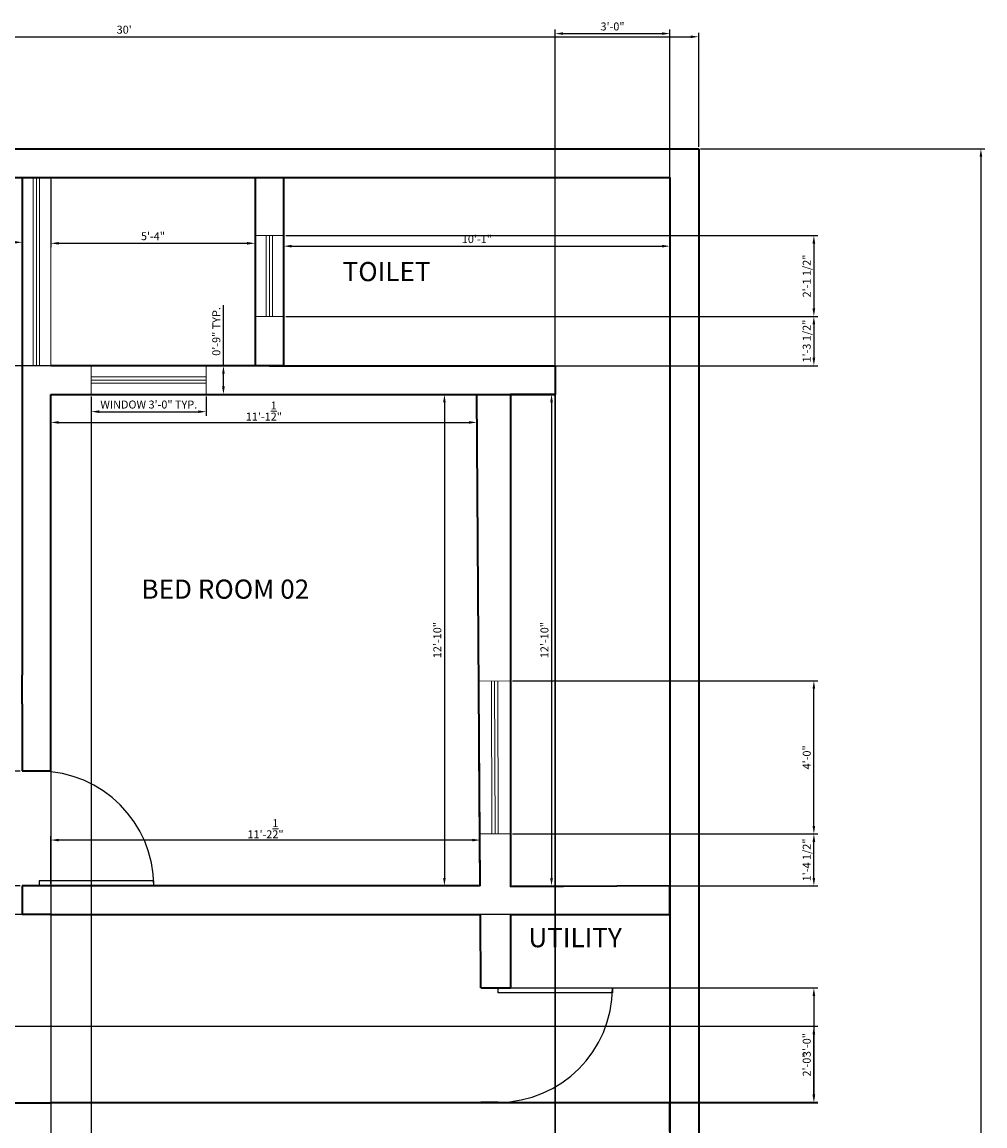
# Model space of a CAD drawing. Units: inches. Extents: x 2178 to 2667, y 1439 to 2239.
# Tile 5 of 5: x 2366 to 2667, y 1891 to 2237. Entities that reach past the tile are written whole.
import ezdxf

# ---------------------------------------------------------------- set-up
doc = ezdxf.new("R2010")
doc.units = ezdxf.units.IN
for name, color, linetype, lineweight in [('A-ANNO-DIMS', 2, 'Continuous', 18), ('A-AREA-IDEN', 7, 'Continuous', 18), ('A-DOOR', 3, 'Continuous', 25), ('A-GLAZ', 4, 'Continuous', 18), ('A-WALL', 7, 'Continuous', 35)]:
    doc.layers.add(name, color=color, linetype=linetype, lineweight=lineweight)
doc.styles.get("Standard").update_dxf_attribs({"font": 'arial.ttf'})
doc.dimstyles.new('Copy of ISO-25', dxfattribs={"dimtxt": 2.5, "dimasz": 2.5, "dimexe": 1.25, "dimexo": 0.625, "dimtad": 1, "dimdec": 1, "dimlunit": 4, "dimtxsty": 'Standard', "dimcen": 2.5, "dimadec": 0, "dimazin": 0, "dimtfac": 1, "dimtdec": 1, "dimtmove": 0, "dimatfit": 3, "dimfxl": 1, "dimarcsym": 0})

# ---------------------------------------------------------------- blocks, each defined once
blk = doc.blocks.new('*D1')
at = {"layer": 'A-ANNO-DIMS', "color": 0, "lineweight": -2, "transparency": 16777216}
for p, q in [((2226.53, 2187.41), (2226.53, 2166.47)), ((2365.53, 2187.41), (2365.53, 2166.47)), ((2229.03, 2167.72), (2363.03, 2167.72))]:
    blk.add_line(p, q, dxfattribs=at)
at = {"layer": 'A-ANNO-DIMS', "color": 0, "transparency": 16777216}
for points in [[(2229.03, 2168.13), (2229.03, 2167.3), (2226.53, 2167.72)], [(2363.03, 2168.13), (2363.03, 2167.3), (2365.53, 2167.72)]]:
    blk.add_solid(points, dxfattribs=at)
at = {"layer": 'Defpoints', "color": 0, "transparency": 16777216}
for p in [(2226.53, 2188.03), (2365.53, 2188.03), (2365.53, 2167.72)]:
    blk.add_point(p, dxfattribs=at)
at = {"layer": 'A-ANNO-DIMS', "color": 0, "transparency": 16777216, "insert": (2296.03, 2169.6), "char_height": 2.5, "attachment_point": 5}
blk.add_mtext('11\'-7"', dxfattribs=at)
blk = doc.blocks.new('*D2')
at = {"layer": 'A-ANNO-DIMS', "color": 0, "lineweight": -2, "transparency": 16777216}
for p, q in [((2374.53, 2187.41), (2374.53, 2166.16)), ((2438.53, 2187.41), (2438.53, 2166.16)), ((2377.03, 2167.41), (2436.03, 2167.41))]:
    blk.add_line(p, q, dxfattribs=at)
at = {"layer": 'A-ANNO-DIMS', "color": 0, "transparency": 16777216}
for points in [[(2377.03, 2167.83), (2377.03, 2166.99), (2374.53, 2167.41)], [(2436.03, 2167.83), (2436.03, 2166.99), (2438.53, 2167.41)]]:
    blk.add_solid(points, dxfattribs=at)
at = {"layer": 'Defpoints', "color": 0, "transparency": 16777216}
for p in [(2374.53, 2188.03), (2438.53, 2188.03), (2438.53, 2167.41)]:
    blk.add_point(p, dxfattribs=at)
at = {"layer": 'A-ANNO-DIMS', "color": 0, "transparency": 16777216, "insert": (2406.53, 2169.31), "char_height": 2.5, "attachment_point": 5}
blk.add_mtext('5\'-4"', dxfattribs=at)
blk = doc.blocks.new('*D3')
at = {"layer": 'A-ANNO-DIMS', "color": 0, "lineweight": -2, "transparency": 16777216}
for p, q in [((2447.53, 2187.41), (2447.53, 2165.26)), ((2568.53, 2187.41), (2568.53, 2165.26)), ((2450.03, 2166.51), (2566.03, 2166.51))]:
    blk.add_line(p, q, dxfattribs=at)
at = {"layer": 'A-ANNO-DIMS', "color": 0, "transparency": 16777216}
for points in [[(2450.03, 2166.93), (2450.03, 2166.09), (2447.53, 2166.51)], [(2566.03, 2166.93), (2566.03, 2166.09), (2568.53, 2166.51)]]:
    blk.add_solid(points, dxfattribs=at)
at = {"layer": 'Defpoints', "color": 0, "transparency": 16777216}
for p in [(2447.53, 2188.03), (2568.53, 2188.03), (2568.53, 2166.51)]:
    blk.add_point(p, dxfattribs=at)
at = {"layer": 'A-ANNO-DIMS', "color": 0, "transparency": 16777216, "insert": (2508.03, 2168.41), "char_height": 2.5, "attachment_point": 5}
blk.add_mtext('10\'-1"', dxfattribs=at)
blk = doc.blocks.new('*D6')
at = {"layer": 'A-ANNO-DIMS', "color": 0, "lineweight": -2, "transparency": 16777216}
for p, q in [((2374.53, 2119.41), (2374.53, 2110.02)), ((2508.03, 2119.41), (2508.03, 2110.02)), ((2377.03, 2111.27), (2505.53, 2111.27))]:
    blk.add_line(p, q, dxfattribs=at)
at = {"layer": 'A-ANNO-DIMS', "color": 0, "transparency": 16777216}
for points in [[(2377.03, 2111.69), (2377.03, 2110.86), (2374.53, 2111.27)], [(2505.53, 2111.69), (2505.53, 2110.86), (2508.03, 2111.27)]]:
    blk.add_solid(points, dxfattribs=at)
at = {"layer": 'Defpoints', "color": 0, "transparency": 16777216}
for p in [(2374.53, 2120.03), (2508.03, 2120.03), (2508.03, 2111.27)]:
    blk.add_point(p, dxfattribs=at)
at = {"layer": 'A-ANNO-DIMS', "color": 0, "transparency": 16777216, "insert": (2441.28, 2114.83), "char_height": 2.5, "attachment_point": 5}
blk.add_mtext('11\'-1{\\H1x;\\S1/2;}"', dxfattribs=at)
blk = doc.blocks.new('*D7')
at = {"layer": 'A-ANNO-DIMS', "color": 0, "lineweight": -2, "transparency": 16777216}
for p, q in [((2507.4, 2120.03), (2496.61, 2120.03)), ((2497.86, 2117.53), (2497.86, 1968.53)), ((2508.44, 1966.03), (2496.61, 1966.03))]:
    blk.add_line(p, q, dxfattribs=at)
at = {"layer": 'A-ANNO-DIMS', "color": 0, "transparency": 16777216}
for points in [[(2497.45, 2117.53), (2498.28, 2117.53), (2497.86, 2120.03)], [(2497.45, 1968.53), (2498.28, 1968.53), (2497.86, 1966.03)]]:
    blk.add_solid(points, dxfattribs=at)
at = {"layer": 'Defpoints', "color": 0, "transparency": 16777216}
for p in [(2508.03, 2120.03), (2497.86, 1966.03), (2509.07, 1966.03)]:
    blk.add_point(p, dxfattribs=at)
at = {"layer": 'A-ANNO-DIMS', "color": 0, "transparency": 16777216, "insert": (2495.96, 2043.03), "char_height": 2.5, "attachment_point": 5, "rotation": 90}
blk.add_mtext('12\'-10"', dxfattribs=at)
blk = doc.blocks.new('*D8')
at = {"layer": 'A-ANNO-DIMS', "color": 0, "lineweight": -2, "transparency": 16777216}
for p, q in [((2374.53, 1966.66), (2374.53, 1981.63)), ((2506.57, 1980.38), (2377.03, 1980.38)), ((2509.07, 1966.66), (2509.07, 1981.63))]:
    blk.add_line(p, q, dxfattribs=at)
at = {"layer": 'A-ANNO-DIMS', "color": 0, "transparency": 16777216}
for points in [[(2377.03, 1980.79), (2377.03, 1979.96), (2374.53, 1980.38)], [(2506.57, 1980.79), (2506.57, 1979.96), (2509.07, 1980.38)]]:
    blk.add_solid(points, dxfattribs=at)
at = {"layer": 'Defpoints', "color": 0, "transparency": 16777216}
for p in [(2374.53, 1980.38), (2374.53, 1966.03), (2509.07, 1966.03)]:
    blk.add_point(p, dxfattribs=at)
at = {"layer": 'A-ANNO-DIMS', "color": 0, "transparency": 16777216, "insert": (2441.8, 1983.93), "char_height": 2.5, "attachment_point": 5}
blk.add_mtext('11\'-2{\\H1x;\\S1/2;}"', dxfattribs=at)
blk = doc.blocks.new('*D9')
at = {"layer": 'A-ANNO-DIMS', "color": 0, "lineweight": -2, "transparency": 16777216}
for p, q in [((2519.15, 2120.03), (2532.68, 2120.03)), ((2531.43, 2117.53), (2531.43, 1968.53)), ((2519.15, 1966.03), (2532.68, 1966.03))]:
    blk.add_line(p, q, dxfattribs=at)
at = {"layer": 'A-ANNO-DIMS', "color": 0, "transparency": 16777216}
for points in [[(2531.01, 2117.53), (2531.85, 2117.53), (2531.43, 2120.03)], [(2531.01, 1968.53), (2531.85, 1968.53), (2531.43, 1966.03)]]:
    blk.add_solid(points, dxfattribs=at)
at = {"layer": 'Defpoints', "color": 0, "transparency": 16777216}
for p in [(2518.53, 2120.03), (2518.53, 1966.03), (2531.43, 1966.03)]:
    blk.add_point(p, dxfattribs=at)
at = {"layer": 'A-ANNO-DIMS', "color": 0, "transparency": 16777216, "insert": (2529.53, 2043.03), "char_height": 2.5, "attachment_point": 5, "rotation": 90}
blk.add_mtext('12\'-10"', dxfattribs=at)
blk = doc.blocks.new('*U23')
for p, q in [((-40, 0), (-40, 6)), ((0, 0), (0, 6))]:
    blk.add_line(p, q)
blk.add_lwpolyline([(0, 0), (0, -40), (-1.75, -40), (-1.75, 0)], close=True)
blk.add_arc((0, 0), 40, 180, 270)
blk = doc.blocks.new('*U22')
for p, q in [((0, 0), (0, 6)), ((40, 0), (40, 6))]:
    blk.add_line(p, q)
blk.add_lwpolyline([(0, 0), (0, -40), (1.75, -40), (1.75, 0)], close=True)
blk.add_arc((0, 0), 40, 270, 0)
blk = doc.blocks.new('*D37')
at = {"layer": 'A-ANNO-DIMS', "color": 0, "lineweight": -2, "transparency": 16777216}
for p, q in [((2364.9, 2001.92), (2358.2, 2001.92)), ((2359.45, 1999.42), (2359.45, 1968.53)), ((2364.9, 1966.03), (2358.2, 1966.03))]:
    blk.add_line(p, q, dxfattribs=at)
at = {"layer": 'A-ANNO-DIMS', "color": 0, "transparency": 16777216}
for points in [[(2359.04, 1999.42), (2359.87, 1999.42), (2359.45, 2001.92)], [(2359.04, 1968.53), (2359.87, 1968.53), (2359.45, 1966.03)]]:
    blk.add_solid(points, dxfattribs=at)
at = {"layer": 'Defpoints', "color": 0, "transparency": 16777216}
for p in [(2365.53, 2001.92), (2359.45, 1966.03), (2365.53, 1966.03)]:
    blk.add_point(p, dxfattribs=at)
at = {"layer": 'A-ANNO-DIMS', "color": 0, "transparency": 16777216, "insert": (2357.55, 1983.98), "char_height": 2.5, "attachment_point": 5, "rotation": 90}
blk.add_mtext("3'", dxfattribs=at)
blk = doc.blocks.new('*D41')
at = {"layer": 'A-ANNO-DIMS', "color": 0, "lineweight": -2, "transparency": 16777216}
for p, q in [((2578.15, 2197.03), (2667.22, 2197.03)), ((2665.97, 2194.53), (2665.97, 1479.53)), ((2578.15, 1477.03), (2667.22, 1477.03))]:
    blk.add_line(p, q, dxfattribs=at)
at = {"layer": 'A-ANNO-DIMS', "color": 0, "transparency": 16777216}
for points in [[(2665.56, 2194.53), (2666.39, 2194.53), (2665.97, 2197.03)], [(2665.56, 1479.53), (2666.39, 1479.53), (2665.97, 1477.03)]]:
    blk.add_solid(points, dxfattribs=at)
at = {"layer": 'Defpoints', "color": 0, "transparency": 16777216}
for p in [(2577.53, 2197.03), (2577.53, 1477.03), (2665.97, 1477.03)]:
    blk.add_point(p, dxfattribs=at)
at = {"layer": 'A-ANNO-DIMS', "color": 0, "transparency": 16777216, "insert": (2664.07, 1837.03), "char_height": 2.5, "attachment_point": 5, "rotation": 90}
blk.add_mtext("60'", dxfattribs=at)
blk = doc.blocks.new('*D42')
at = {"layer": 'A-ANNO-DIMS', "color": 0, "lineweight": -2, "transparency": 16777216}
for p, q in [((2217.53, 2197.66), (2217.53, 2233.38)), ((2220.03, 2232.13), (2575.03, 2232.13)), ((2577.53, 2197.66), (2577.53, 2233.38))]:
    blk.add_line(p, q, dxfattribs=at)
at = {"layer": 'A-ANNO-DIMS', "color": 0, "transparency": 16777216}
for points in [[(2220.03, 2232.54), (2220.03, 2231.71), (2217.53, 2232.13)], [(2575.03, 2232.54), (2575.03, 2231.71), (2577.53, 2232.13)]]:
    blk.add_solid(points, dxfattribs=at)
at = {"layer": 'Defpoints', "color": 0, "transparency": 16777216}
for p in [(2577.53, 2232.13), (2217.53, 2197.03), (2577.53, 2197.03)]:
    blk.add_point(p, dxfattribs=at)
at = {"layer": 'A-ANNO-DIMS', "color": 0, "transparency": 16777216, "insert": (2397.53, 2234.03), "char_height": 2.5, "attachment_point": 5}
blk.add_mtext("30'", dxfattribs=at)
blk = doc.blocks.new('WIN-36IN')
for p, q in [((0, 0), (0, 9)), ((36, 9), (36, 0)), ((0, 5.5), (36, 5.5)), ((0, 4.5), (36, 4.5)), ((0, 3.5), (36, 3.5)), ((36, 0), (0, 0))]:
    blk.add_line(p, q)
blk = doc.blocks.new('*D46')
at = {"layer": 'A-ANNO-DIMS', "color": 0, "lineweight": -2, "transparency": 16777216}
for p, q in [((2387.22, 2119.41), (2387.22, 2113.38)), ((2423.22, 2119.41), (2423.22, 2113.38)), ((2389.72, 2114.63), (2420.72, 2114.63))]:
    blk.add_line(p, q, dxfattribs=at)
at = {"layer": 'A-ANNO-DIMS', "color": 0, "transparency": 16777216}
for points in [[(2389.72, 2115.05), (2389.72, 2114.22), (2387.22, 2114.63)], [(2420.72, 2115.05), (2420.72, 2114.22), (2423.22, 2114.63)]]:
    blk.add_solid(points, dxfattribs=at)
at = {"layer": 'Defpoints', "color": 0, "transparency": 16777216}
for p in [(2387.22, 2120.03), (2423.22, 2120.03), (2423.22, 2114.63)]:
    blk.add_point(p, dxfattribs=at)
at = {"layer": 'A-ANNO-DIMS', "color": 0, "transparency": 16777216, "insert": (2405.22, 2116.55), "char_height": 2.5, "attachment_point": 5}
blk.add_mtext('WINDOW 3\'-0" TYP.', dxfattribs=at)
blk = doc.blocks.new('*D47')
at = {"layer": 'A-ANNO-DIMS', "color": 0, "lineweight": -2, "transparency": 16777216}
for p, q in [((2428.62, 2129.03), (2428.62, 2148.02)), ((2423.84, 2129.03), (2429.87, 2129.03)), ((2428.62, 2122.53), (2428.62, 2126.53)), ((2423.84, 2120.03), (2429.87, 2120.03))]:
    blk.add_line(p, q, dxfattribs=at)
at = {"layer": 'A-ANNO-DIMS', "color": 0, "transparency": 16777216}
for points in [[(2428.2, 2126.53), (2429.03, 2126.53), (2428.62, 2129.03)], [(2428.2, 2122.53), (2429.03, 2122.53), (2428.62, 2120.03)]]:
    blk.add_solid(points, dxfattribs=at)
at = {"layer": 'Defpoints', "color": 0, "transparency": 16777216}
for p in [(2423.22, 2129.03), (2428.62, 2129.03), (2423.22, 2120.03)]:
    blk.add_point(p, dxfattribs=at)
at = {"layer": 'A-ANNO-DIMS', "color": 0, "transparency": 16777216, "insert": (2426.71, 2139.78), "char_height": 2.5, "attachment_point": 5, "rotation": 90}
blk.add_mtext('0\'-9" TYP.', dxfattribs=at)
blk = doc.blocks.new('*D48')
at = {"layer": 'A-ANNO-DIMS', "color": 0, "lineweight": -2, "transparency": 16777216}
for p, q in [((2437.9, 2188.03), (2180.18, 2188.03)), ((2181.43, 2185.53), (2181.43, 2131.53)), ((2437.9, 2129.03), (2180.18, 2129.03))]:
    blk.add_line(p, q, dxfattribs=at)
at = {"layer": 'A-ANNO-DIMS', "color": 0, "transparency": 16777216}
for points in [[(2181.01, 2185.53), (2181.84, 2185.53), (2181.43, 2188.03)], [(2181.01, 2131.53), (2181.84, 2131.53), (2181.43, 2129.03)]]:
    blk.add_solid(points, dxfattribs=at)
at = {"layer": 'Defpoints', "color": 0, "transparency": 16777216}
for p in [(2438.53, 2188.03), (2181.43, 2129.03), (2438.53, 2129.03)]:
    blk.add_point(p, dxfattribs=at)
at = {"layer": 'A-ANNO-DIMS', "color": 0, "transparency": 16777216, "insert": (2179.55, 2158.53), "char_height": 2.5, "attachment_point": 5, "rotation": 90}
blk.add_mtext('4\'-11"', dxfattribs=at)
blk = doc.blocks.new('*D49')
at = {"layer": 'A-ANNO-DIMS', "color": 0, "lineweight": -2, "transparency": 16777216}
for p, q in [((2567.9, 1957.03), (2180.18, 1957.03)), ((2181.43, 1954.53), (2181.43, 1900.53)), ((2567.9, 1898.03), (2180.18, 1898.03))]:
    blk.add_line(p, q, dxfattribs=at)
at = {"layer": 'A-ANNO-DIMS', "color": 0, "transparency": 16777216}
for points in [[(2181.01, 1954.53), (2181.84, 1954.53), (2181.43, 1957.03)], [(2181.01, 1900.53), (2181.84, 1900.53), (2181.43, 1898.03)]]:
    blk.add_solid(points, dxfattribs=at)
at = {"layer": 'Defpoints', "color": 0, "transparency": 16777216}
for p in [(2568.53, 1957.03), (2181.43, 1898.03), (2568.53, 1898.03)]:
    blk.add_point(p, dxfattribs=at)
at = {"layer": 'A-ANNO-DIMS', "color": 0, "transparency": 16777216, "insert": (2179.55, 1927.53), "char_height": 2.5, "attachment_point": 5, "rotation": 90}
blk.add_mtext('4\'-11"', dxfattribs=at)
blk = doc.blocks.new('*D55')
at = {"layer": 'A-ANNO-DIMS', "color": 0, "lineweight": -2, "transparency": 16777216}
for p, q in [((2519.15, 1982.29), (2614.88, 1982.29)), ((2613.63, 1968.53), (2613.63, 1979.79)), ((2519.15, 1966.03), (2614.88, 1966.03))]:
    blk.add_line(p, q, dxfattribs=at)
at = {"layer": 'A-ANNO-DIMS', "color": 0, "transparency": 16777216}
for points in [[(2613.21, 1979.79), (2614.04, 1979.79), (2613.63, 1982.29)], [(2613.21, 1968.53), (2614.04, 1968.53), (2613.63, 1966.03)]]:
    blk.add_solid(points, dxfattribs=at)
at = {"layer": 'Defpoints', "color": 0, "transparency": 16777216}
for p in [(2518.53, 1982.29), (2613.63, 1982.29), (2518.53, 1966.03)]:
    blk.add_point(p, dxfattribs=at)
at = {"layer": 'A-ANNO-DIMS', "color": 0, "transparency": 16777216, "insert": (2611.71, 1974.16), "char_height": 2.5, "attachment_point": 5, "rotation": 90}
blk.add_mtext('1\'-4 1/2"', dxfattribs=at)
blk = doc.blocks.new('*D56')
at = {"layer": 'A-ANNO-DIMS', "color": 0, "lineweight": -2, "transparency": 16777216}
for p, q in [((2519.15, 2030.29), (2614.88, 2030.29)), ((2613.63, 1984.79), (2613.63, 2027.79)), ((2519.15, 1982.29), (2614.88, 1982.29))]:
    blk.add_line(p, q, dxfattribs=at)
at = {"layer": 'A-ANNO-DIMS', "color": 0, "transparency": 16777216}
for points in [[(2613.21, 2027.79), (2614.04, 2027.79), (2613.63, 2030.29)], [(2613.21, 1984.79), (2614.04, 1984.79), (2613.63, 1982.29)]]:
    blk.add_solid(points, dxfattribs=at)
at = {"layer": 'Defpoints', "color": 0, "transparency": 16777216}
for p in [(2518.53, 2030.29), (2613.63, 2030.29), (2518.53, 1982.29)]:
    blk.add_point(p, dxfattribs=at)
at = {"layer": 'A-ANNO-DIMS', "color": 0, "transparency": 16777216, "insert": (2611.72, 2006.29), "char_height": 2.5, "attachment_point": 5, "rotation": 90}
blk.add_mtext('4\'-0"', dxfattribs=at)
blk = doc.blocks.new('*D57')
at = {"layer": 'A-ANNO-DIMS', "color": 0, "lineweight": -2, "transparency": 16777216}
for p, q in [((2374.53, 2119.41), (2374.53, 1439.68)), ((2387.22, 2119.41), (2387.22, 1439.68)), ((2377.03, 1440.93), (2384.72, 1440.93)), ((2387.22, 1440.93), (2403.2, 1440.93))]:
    blk.add_line(p, q, dxfattribs=at)
at = {"layer": 'A-ANNO-DIMS', "color": 0, "transparency": 16777216}
for points in [[(2377.03, 1441.35), (2377.03, 1440.52), (2374.53, 1440.93)], [(2384.72, 1441.35), (2384.72, 1440.52), (2387.22, 1440.93)]]:
    blk.add_solid(points, dxfattribs=at)
at = {"layer": 'Defpoints', "color": 0, "transparency": 16777216}
for p in [(2374.53, 2120.03), (2387.22, 2120.03), (2387.22, 1440.93)]:
    blk.add_point(p, dxfattribs=at)
at = {"layer": 'A-ANNO-DIMS', "color": 0, "transparency": 16777216, "insert": (2396.46, 1442.85), "char_height": 2.5, "attachment_point": 5}
blk.add_mtext('1\'-0 1/2"', dxfattribs=at)
blk = doc.blocks.new('*D59')
at = {"layer": 'A-ANNO-DIMS', "color": 0, "lineweight": -2, "transparency": 16777216}
for p, q in [((2448.15, 2169.84), (2614.88, 2169.84)), ((2613.63, 2167.34), (2613.63, 2146.98)), ((2448.15, 2144.48), (2614.88, 2144.48))]:
    blk.add_line(p, q, dxfattribs=at)
at = {"layer": 'A-ANNO-DIMS', "color": 0, "transparency": 16777216}
for points in [[(2613.21, 2167.34), (2614.04, 2167.34), (2613.63, 2169.84)], [(2613.21, 2146.98), (2614.04, 2146.98), (2613.63, 2144.48)]]:
    blk.add_solid(points, dxfattribs=at)
at = {"layer": 'Defpoints', "color": 0, "transparency": 16777216}
for p in [(2447.53, 2169.84), (2447.53, 2144.48), (2613.63, 2144.48)]:
    blk.add_point(p, dxfattribs=at)
at = {"layer": 'A-ANNO-DIMS', "color": 0, "transparency": 16777216, "insert": (2611.71, 2157.16), "char_height": 2.5, "attachment_point": 5, "rotation": 90}
blk.add_mtext('2\'-1 1/2"', dxfattribs=at)
blk = doc.blocks.new('*D60')
at = {"layer": 'A-ANNO-DIMS', "color": 0, "lineweight": -2, "transparency": 16777216}
for p, q in [((2448.15, 2144.48), (2614.88, 2144.48)), ((2613.63, 2141.98), (2613.63, 2131.53)), ((2448.15, 2129.03), (2614.88, 2129.03))]:
    blk.add_line(p, q, dxfattribs=at)
at = {"layer": 'A-ANNO-DIMS', "color": 0, "transparency": 16777216}
for points in [[(2613.21, 2141.98), (2614.04, 2141.98), (2613.63, 2144.48)], [(2613.21, 2131.53), (2614.04, 2131.53), (2613.63, 2129.03)]]:
    blk.add_solid(points, dxfattribs=at)
at = {"layer": 'Defpoints', "color": 0, "transparency": 16777216}
for p in [(2447.53, 2144.48), (2447.53, 2129.03), (2613.63, 2129.03)]:
    blk.add_point(p, dxfattribs=at)
at = {"layer": 'A-ANNO-DIMS', "color": 0, "transparency": 16777216, "insert": (2611.71, 2136.76), "char_height": 2.5, "attachment_point": 5, "rotation": 90}
blk.add_mtext('1\'-3 1/2"', dxfattribs=at)
blk = doc.blocks.new('*D68')
at = {"layer": 'A-ANNO-DIMS', "color": 0, "lineweight": -2, "transparency": 16777216}
for p, q in [((2321.15, 1922.03), (2614.88, 1922.03)), ((2613.63, 1900.53), (2613.63, 1919.53)), ((2321.15, 1898.03), (2614.88, 1898.03))]:
    blk.add_line(p, q, dxfattribs=at)
at = {"layer": 'A-ANNO-DIMS', "color": 0, "transparency": 16777216}
for points in [[(2613.21, 1919.53), (2614.04, 1919.53), (2613.63, 1922.03)], [(2613.21, 1900.53), (2614.04, 1900.53), (2613.63, 1898.03)]]:
    blk.add_solid(points, dxfattribs=at)
at = {"layer": 'Defpoints', "color": 0, "transparency": 16777216}
for p in [(2320.53, 1922.03), (2613.63, 1922.03), (2320.53, 1898.03)]:
    blk.add_point(p, dxfattribs=at)
at = {"layer": 'A-ANNO-DIMS', "color": 0, "transparency": 16777216, "insert": (2611.72, 1910.03), "char_height": 2.5, "attachment_point": 5, "rotation": 90}
blk.add_mtext('2\'-0"', dxfattribs=at)
blk = doc.blocks.new('*D70')
at = {"layer": 'A-ANNO-DIMS', "color": 0, "lineweight": -2, "transparency": 16777216}
for p, q in [((2532.53, 1798.37), (2532.53, 2234.38)), ((2535.03, 2233.13), (2566.03, 2233.13)), ((2568.53, 1798.37), (2568.53, 2234.38))]:
    blk.add_line(p, q, dxfattribs=at)
at = {"layer": 'A-ANNO-DIMS', "color": 0, "transparency": 16777216}
for points in [[(2535.03, 2233.55), (2535.03, 2232.72), (2532.53, 2233.13)], [(2566.03, 2233.55), (2566.03, 2232.72), (2568.53, 2233.13)]]:
    blk.add_solid(points, dxfattribs=at)
at = {"layer": 'Defpoints', "color": 0, "transparency": 16777216}
for p in [(2568.53, 2233.13), (2532.53, 1797.74), (2568.53, 1797.74)]:
    blk.add_point(p, dxfattribs=at)
at = {"layer": 'A-ANNO-DIMS', "color": 0, "transparency": 16777216, "insert": (2550.53, 2235.04), "char_height": 2.5, "attachment_point": 5}
blk.add_mtext('3\'-0"', dxfattribs=at)
blk = doc.blocks.new('*D71')
at = {"layer": 'A-ANNO-DIMS', "color": 0, "lineweight": -2, "transparency": 16777216}
for p, q in [((2519.15, 1934.03), (2614.88, 1934.03)), ((2613.63, 1931.53), (2613.63, 1900.69)), ((2515.28, 1898.19), (2614.88, 1898.19))]:
    blk.add_line(p, q, dxfattribs=at)
at = {"layer": 'A-ANNO-DIMS', "color": 0, "transparency": 16777216}
for points in [[(2613.21, 1931.53), (2614.04, 1931.53), (2613.63, 1934.03)], [(2613.21, 1900.69), (2614.04, 1900.69), (2613.63, 1898.19)]]:
    blk.add_solid(points, dxfattribs=at)
at = {"layer": 'Defpoints', "color": 0, "transparency": 16777216}
for p in [(2518.53, 1934.03), (2514.66, 1898.19), (2613.63, 1898.19)]:
    blk.add_point(p, dxfattribs=at)
at = {"layer": 'A-ANNO-DIMS', "color": 0, "transparency": 16777216, "insert": (2611.72, 1916.11), "char_height": 2.5, "attachment_point": 5, "rotation": 90}
blk.add_mtext('3\'-0"', dxfattribs=at)
blk = doc.blocks.new('*D73')
at = {"layer": 'A-ANNO-DIMS', "color": 0, "lineweight": -2, "transparency": 16777216}
for p, q in [((2568.53, 2187.41), (2568.53, 1439.68)), ((2532.53, 2128.41), (2532.53, 1439.68)), ((2535.03, 1440.93), (2566.03, 1440.93))]:
    blk.add_line(p, q, dxfattribs=at)
at = {"layer": 'A-ANNO-DIMS', "color": 0, "transparency": 16777216}
for points in [[(2535.03, 1441.35), (2535.03, 1440.52), (2532.53, 1440.93)], [(2566.03, 1441.35), (2566.03, 1440.52), (2568.53, 1440.93)]]:
    blk.add_solid(points, dxfattribs=at)
at = {"layer": 'Defpoints', "color": 0, "transparency": 16777216}
for p in [(2568.53, 2188.03), (2532.53, 2129.03), (2568.53, 1440.93)]:
    blk.add_point(p, dxfattribs=at)
at = {"layer": 'A-ANNO-DIMS', "color": 0, "transparency": 16777216, "insert": (2550.53, 1442.84), "char_height": 2.5, "attachment_point": 5}
blk.add_mtext('3\'-0"', dxfattribs=at)

msp = doc.modelspace()

# ---------------------------------------------------------------- linework, layer by layer
at = {"layer": 'A-GLAZ'}
for p, q in [((2369.03, 2129.03), (2369.03, 2188.03)), ((2370.03, 2129.03), (2370.03, 2188.03)), ((2371.03, 2129.03), (2371.03, 2188.03)), ((2374.53, 2129.03), (2374.53, 2188.03)), ((2438.53, 2169.84), (2447.53, 2169.84)), ((2442.03, 2169.84), (2442.03, 2144.48)), ((2443.03, 2169.84), (2443.03, 2144.48)), ((2444.03, 2169.84), (2444.03, 2144.48)), ((2447.53, 2169.84), (2447.53, 2144.48)), ((2447.53, 2144.48), (2438.53, 2144.48)), ((2518.53, 2030.29), (2508.63, 2030.22)), ((2512.58, 2030.25), (2512.74, 1982.28)), ((2513.58, 2030.25), (2513.74, 1982.29)), ((2514.58, 2030.26), (2514.74, 1982.29)), ((2518.53, 1982.29), (2518.53, 2030.29)), ((2514.65, 2009.04), (2514.65, 2009.03)), ((2508.96, 1982.29), (2518.53, 1982.29))]:
    msp.add_line(p, q, dxfattribs=at)
msp.add_lwpolyline([(2374.53, 2129.03), (2365.53, 2129.03)], dxfattribs=at)
at = {"layer": 'A-WALL'}
for p, q in [((2217.53, 2197.03), (2577.53, 2197.03)), ((2577.53, 2197.03), (2577.53, 1477.03)), ((2226.53, 2188.03), (2568.53, 2188.03)), ((2226.53, 2188.03), (2365.53, 2188.03)), ((2365.53, 2188.03), (2365.53, 2032.03)), ((2374.53, 2188.03), (2438.53, 2188.03)), ((2438.53, 2188.03), (2438.53, 2129.03)), ((2438.53, 2188.03), (2438.53, 2169.84)), ((2447.53, 2129.03), (2447.53, 2188.03)), ((2568.53, 2188.03), (2568.53, 1749.74)), ((2438.53, 2129.03), (2374.53, 2129.03)), ((2438.53, 2129.03), (2423.22, 2129.03)), ((2447.53, 2129.03), (2438.53, 2129.03)), ((2443.03, 2129.03), (2447.53, 2129.03)), ((2447.53, 2129.03), (2532.53, 2129.03)), ((2532.53, 2129.03), (2532.53, 2120.03)), ((2374.53, 2023.03), (2374.53, 2120.03)), ((2374.53, 2120.03), (2438.53, 2120.03)), ((2438.53, 2120.03), (2447.53, 2120.03)), ((2447.53, 2120.03), (2532.53, 2120.03)), ((2509.07, 1966.03), (2508.03, 2120.03)), ((2532.53, 2120.03), (2518.53, 2120.03)), ((2518.53, 2120.03), (2518.53, 1965.7)), ((2518.53, 2120.03), (2518.53, 1966.03)), ((2365.53, 2023.03), (2365.53, 2032.03)), ((2365.53, 2023.03), (2365.53, 2002.03)), ((2374.53, 2002.03), (2374.53, 2023.03)), ((2509.07, 1966.03), (2508.78, 2009.03)), ((2365.53, 2002.03), (2374.53, 2002.03)), ((2509.07, 1966.03), (2508.96, 1982.29)), ((2365.53, 1966.03), (2365.53, 1957.03)), ((2374.53, 1966.03), (2365.53, 1966.03)), ((2365.53, 1966.03), (2365.53, 1957.03)), ((2509.07, 1966.03), (2374.53, 1966.03)), ((2568.53, 1966.03), (2518.53, 1965.7)), ((2568.53, 1957.03), (2568.53, 1966.03)), ((2374.53, 1957.03), (2365.53, 1957.03)), ((2374.53, 1957.03), (2509.13, 1957.03)), ((2509.28, 1934.03), (2509.13, 1957.03)), ((2518.53, 1957.03), (2568.53, 1957.03)), ((2518.53, 1957.03), (2518.53, 1934.03)), ((2509.53, 1934.03), (2509.28, 1934.03)), ((2509.53, 1934.03), (2518.53, 1934.03)), ((2226.53, 1898.03), (2365.53, 1898.03)), ((2365.53, 1898.03), (2374.53, 1898.03)), ((2568.53, 1898.03), (2374.53, 1898.03)), ((2518.53, 1898.03), (2509.53, 1898.03)), ((2568.53, 1889.03), (2568.53, 1898.03))]:
    msp.add_line(p, q, dxfattribs=at)

# ---------------------------------------------------------------- block references
at = {"layer": 'A-DOOR', "rotation": 90}
for name, p, xscale, yscale, zscale in [('*U22', (2370.91, 1966.03), 0.8971499256419678, 0.8971499256419678, 0.8971499256419678), ('*U23', (2514.66, 1934.03), 0.896210211266654, 0.896210211266654, 0.896210211266654)]:
    msp.add_blockref(name, p, dxfattribs=dict(at, xscale=xscale, yscale=yscale, zscale=zscale))
at = {"layer": 'A-GLAZ'}
msp.add_blockref('WIN-36IN', (2387.22, 2120.03), dxfattribs=at)

# ---------------------------------------------------------------- texts
at = {"layer": 'A-AREA-IDEN'}
for s, p in [('TOILET', (2465.97, 2155.54)), ('BED ROOM 02', (2402.92, 2056.02)), ('UTILITY', (2524.16, 1946.79))]:
    msp.add_text(s, height=6, dxfattribs=at).set_placement(p)

# ---------------------------------------------------------------- dimensions: what is measured, and where the dimension line sits
at = {"layer": 'A-ANNO-DIMS'}
for base, p1, p2, override, picture, middle in [((2577.53, 2232.13), (2217.53, 2197.03), (2577.53, 2197.03), {"dimclrd": 0, "dimclre": 0, "dimclrt": 0}, '*D42', (2397.53, 2234.03)), ((2568.53, 2233.13), (2532.53, 1797.74), (2568.53, 1797.74), {"dimdec": 1, "dimlfac": 1, "dimrnd": 0, "dimzin": 1, "dimdsep": 46, "dimlunit": 4, "dimfrac": 2}, '*D70', (2550.53, 2235.04)), ((2365.53, 2167.72), (2226.53, 2188.03), (2365.53, 2188.03), {"dimclrd": 0, "dimclre": 0, "dimclrt": 0}, '*D1', (2296.03, 2169.6)), ((2438.53, 2167.41), (2374.53, 2188.03), (2438.53, 2188.03), {"dimclrd": 0, "dimclre": 0, "dimclrt": 0}, '*D2', (2406.53, 2169.31)), ((2568.53, 2166.51), (2447.53, 2188.03), (2568.53, 2188.03), {"dimclrd": 0, "dimclre": 0, "dimclrt": 0}, '*D3', (2508.03, 2168.41)), ((2568.53, 1440.93), (2532.53, 2129.03), (2568.53, 2188.03), {"dimdec": 1, "dimlfac": 1, "dimrnd": 0, "dimzin": 1, "dimdsep": 46, "dimlunit": 4, "dimfrac": 2}, '*D73', (2550.53, 1442.84)), ((2508.03, 2111.27), (2374.53, 2120.03), (2508.03, 2120.03), {"dimclrd": 0, "dimclre": 0, "dimclrt": 0}, '*D6', (2441.28, 2114.83)), ((2387.22, 1440.93), (2374.53, 2120.03), (2387.22, 2120.03), {"dimdec": 1, "dimlfac": 1, "dimrnd": 0, "dimzin": 1, "dimdsep": 46, "dimlunit": 4, "dimfrac": 2}, '*D57', (2396.46, 1442.85)), ((2374.53, 1980.38), (2509.07, 1966.03), (2374.53, 1966.03), {"dimclrd": 0, "dimclre": 0, "dimclrt": 0}, '*D8', (2441.8, 1983.93))]:
    dim = msp.add_linear_dim(base=base, p1=p1, p2=p2, dimstyle='Copy of ISO-25', override=override, dxfattribs=at)
    dim.commit()
    dim.dimension.update_dxf_attribs({"geometry": picture, "text_midpoint": middle})
for base, p1, p2, override, picture, middle in [((2665.97, 1477.03), (2577.53, 2197.03), (2577.53, 1477.03), {"dimclrd": 0, "dimclre": 0, "dimclrt": 0}, '*D41', (2664.07, 1837.03)), ((2181.43, 2129.03), (2438.53, 2188.03), (2438.53, 2129.03), {"dimdec": 1, "dimlfac": 1, "dimrnd": 0, "dimzin": 1, "dimdsep": 46, "dimlunit": 4, "dimfrac": 2}, '*D48', (2179.55, 2158.53)), ((2613.63, 2144.48), (2447.53, 2169.84), (2447.53, 2144.48), {"dimdec": 1, "dimlfac": 1, "dimrnd": 0, "dimzin": 1, "dimdsep": 46, "dimlunit": 4, "dimfrac": 2}, '*D59', (2611.71, 2157.16)), ((2613.6256, 2129.0346), (2447.5256, 2144.4827), (2447.5256, 2129.0346), {"dimdec": 1, "dimlfac": 1, "dimrnd": 0, "dimzin": 1, "dimdsep": 46, "dimlunit": 4, "dimfrac": 2}, '*D60', (2611.7071, 2136.7586)), ((2497.86, 1966.03), (2508.03, 2120.03), (2509.07, 1966.03), {"dimclrd": 0, "dimclre": 0, "dimclrt": 0}, '*D7', (2495.96, 2043.03)), ((2531.43, 1966.03), (2518.53, 2120.03), (2518.53, 1966.03), {"dimclrd": 0, "dimclre": 0, "dimclrt": 0}, '*D9', (2529.53, 2043.03)), ((2613.63, 2030.29), (2518.53, 1982.29), (2518.53, 2030.29), {"dimdec": 1, "dimlfac": 1, "dimrnd": 0, "dimzin": 1, "dimdsep": 46, "dimlunit": 4, "dimfrac": 2}, '*D56', (2611.72, 2006.29)), ((2359.45, 1966.03), (2365.53, 2001.92), (2365.53, 1966.03), {"dimclrd": 0, "dimclre": 0, "dimclrt": 0}, '*D37', (2357.55, 1983.98)), ((2613.63, 1982.29), (2518.53, 1966.03), (2518.53, 1982.29), {"dimdec": 1, "dimlfac": 1, "dimrnd": 0, "dimzin": 1, "dimdsep": 46, "dimlunit": 4, "dimfrac": 2}, '*D55', (2611.71, 1974.16)), ((2181.43, 1898.03), (2568.53, 1957.03), (2568.53, 1898.03), {"dimdec": 1, "dimlfac": 1, "dimrnd": 0, "dimzin": 1, "dimdsep": 46, "dimlunit": 4, "dimfrac": 2}, '*D49', (2179.55, 1927.53)), ((2613.63, 1898.19), (2518.53, 1934.03), (2514.66, 1898.19), {"dimdec": 1, "dimlfac": 1, "dimrnd": 0, "dimzin": 1, "dimdsep": 46, "dimlunit": 4, "dimfrac": 2}, '*D71', (2611.72, 1916.11)), ((2613.63, 1922.03), (2320.53, 1898.03), (2320.53, 1922.03), {"dimdec": 1, "dimlfac": 1, "dimrnd": 0, "dimzin": 1, "dimdsep": 46, "dimlunit": 4, "dimfrac": 2}, '*D68', (2611.72, 1910.03))]:
    dim = msp.add_linear_dim(base=base, p1=p1, p2=p2, angle=90, dimstyle='Copy of ISO-25', override=override, dxfattribs=at)
    dim.commit()
    dim.dimension.update_dxf_attribs({"geometry": picture, "text_midpoint": middle})
dim = msp.add_linear_dim(base=(2428.62, 2129.03), p1=(2423.22, 2120.03), p2=(2423.22, 2129.03), angle=90, text='<> TYP.', dimstyle='Copy of ISO-25', override={"dimdec": 1, "dimlfac": 1, "dimrnd": 0, "dimzin": 1, "dimdsep": 46, "dimlunit": 4, "dimfrac": 2}, dxfattribs=at)
dim.commit()
dim.dimension.update_dxf_attribs({"geometry": '*D47', "text_midpoint": (2426.71, 2139.78)})
dim = msp.add_linear_dim(base=(2423.22, 2114.63), p1=(2387.22, 2120.03), p2=(2423.22, 2120.03), text='WINDOW <> TYP.', dimstyle='Copy of ISO-25', override={"dimdec": 1, "dimlfac": 1, "dimrnd": 0, "dimzin": 1, "dimdsep": 46, "dimlunit": 4, "dimfrac": 2}, dxfattribs=at)
dim.commit()
dim.dimension.update_dxf_attribs({"geometry": '*D46', "text_midpoint": (2405.22, 2116.55)})

doc.saveas('drawing.dxf')
